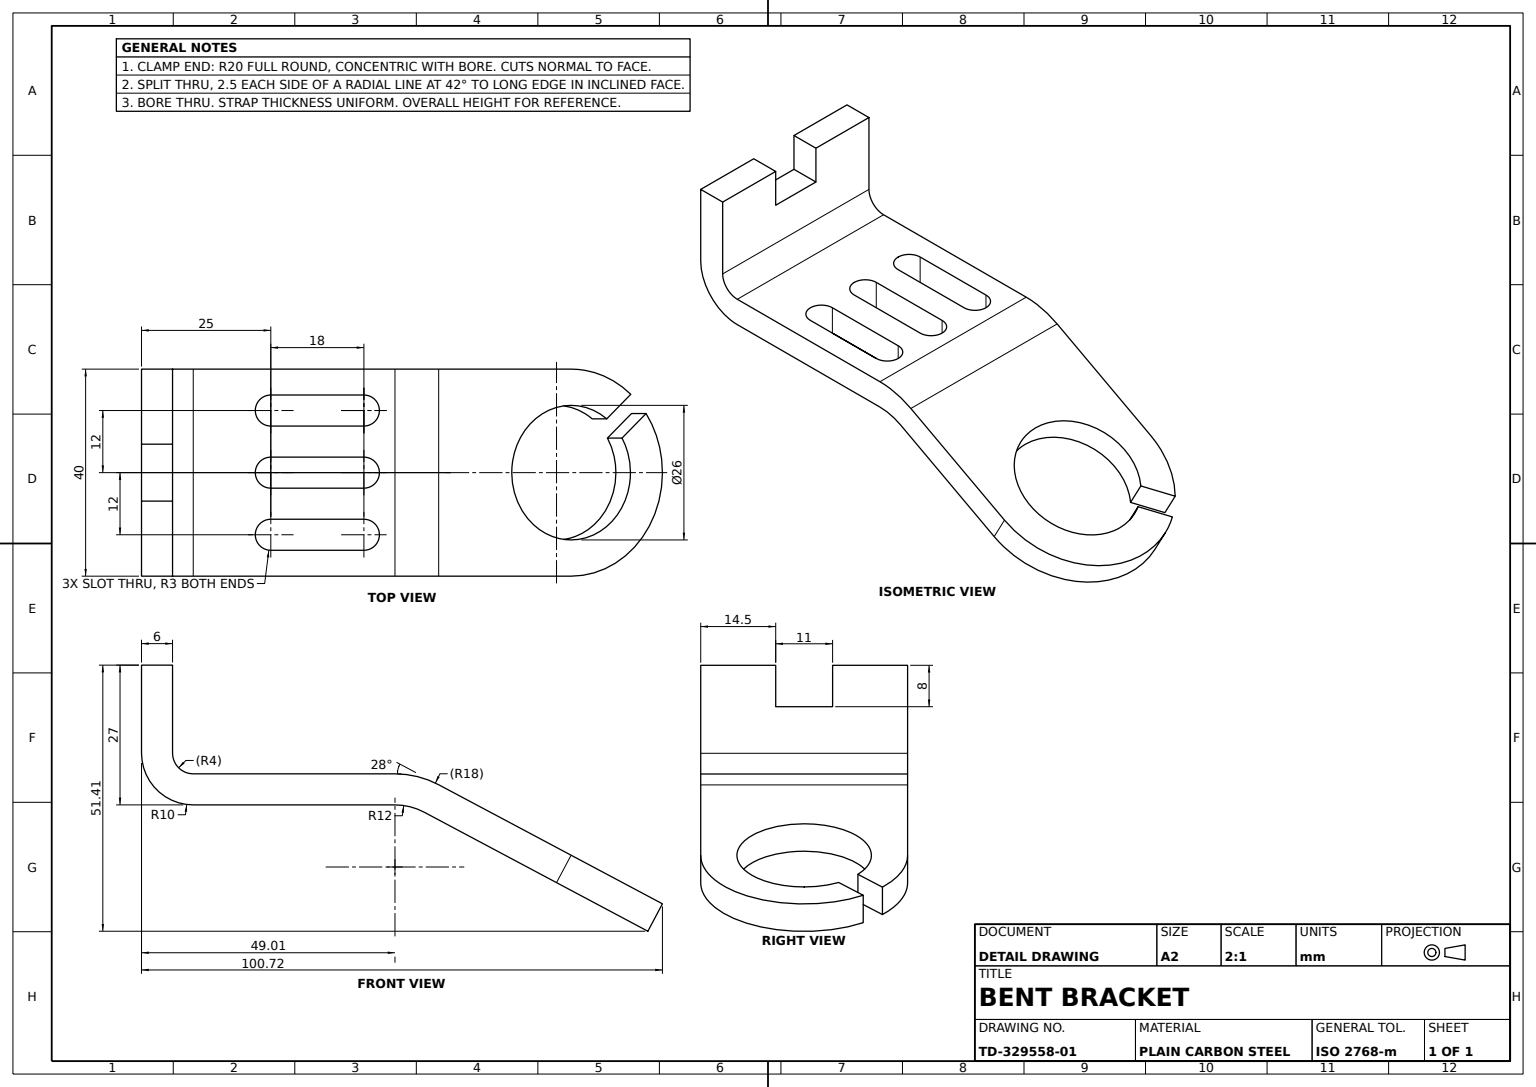
SolidWorks part; units mm, degrees
material "Plain Carbon Steel"
ref_plane "Front Plane" through (0, 0, 0) normal (0, 0, 1) x (1, 0, 0)
ref_plane "Top Plane" through (0, 0, 0) normal (0, 1, 0) x (1, 0, 0)
ref_plane "Right Plane" through (0, 0, 0) normal (1, 0, 0) x (0, 0, -1)
sketch "Strap Profile Sketch" plane through (0, 0, 0) normal (0, 0, 1) x (1, 0, 0)
  line L0 (0, 27) -> (0, 10)
  line L1 (10, 0) -> (49.0081, 0)
  line L2 (54.6417, -1.4046) -> (102, -26.5855)
  line L3 (6, 27) -> (6, 10)
  line L4 (10, 6) -> (49.0081, 6)
  line L5 (57.4586, 3.8931) -> (104.8168, -21.2878)
  line L6 (0, 27) -> (6, 27)
  line L7 (104.8168, -21.2878) -> (102, -26.5855)
  arc A0 (0, 10) -> (10, 0) centre (10, 10) ccw
  arc A1 (49.0081, 0) -> (54.6417, -1.4046) centre (49.0081, -12) cw
  arc A2 (6, 10) -> (10, 6) centre (10, 10) ccw
  arc A3 (49.0081, 6) -> (57.4586, 3.8931) centre (49.0081, -12) cw
  point P7 (0, 0)
  point P10 (52, 0)
  dimension "D4" = 10
  dimension "D5" = 12
  dimension "D1" = 27
  dimension "D2" = 52
  dimension "D3" = 50
  dimension "D6" = 28
  dimension "D7" = 6
extrude "Bent Strap Body" add sketch "Strap Profile Sketch" along normal blind 40
sketch "Slots Sketch" plane through (0, 6, 0) normal (0, 1, 0) x (1, 0, 0)
  line L0 (25, -20) -> (43, -20) construction
  line L1 (25, -17) -> (43, -17)
  line L2 (25, -23) -> (43, -23)
  line L3 (0, -40) -> (0, 0) construction
  line L4 (25, -8) -> (43, -8) construction
  line L5 (25, -5) -> (43, -5)
  line L6 (25, -11) -> (43, -11)
  line L7 (25, -32) -> (43, -32) construction
  line L8 (25, -29) -> (43, -29)
  line L9 (25, -35) -> (43, -35)
  line L10 (49.0081, 0) -> (10, 0) construction
  arc A0 (25, -17) -> (25, -23) centre (25, -20) ccw
  arc A1 (43, -23) -> (43, -17) centre (43, -20) ccw
  arc A2 (25, -5) -> (25, -11) centre (25, -8) ccw
  arc A3 (43, -11) -> (43, -5) centre (43, -8) ccw
  arc A4 (25, -29) -> (25, -35) centre (25, -32) ccw
  arc A5 (43, -35) -> (43, -29) centre (43, -32) ccw
  point P2 (34, -20)
  point P11 (34, -8)
  point P18 (34, -32)
  dimension "D1" = 18
  dimension "D2" = 25
  dimension "D3" = 6
  dimension "D4" = 18
  dimension "D5" = 25
  dimension "D6" = 12
  dimension "D7" = 6
  dimension "D8" = 6
  dimension "D9" = 18
  dimension "D10" = 25
  dimension "D11" = 12
  dimension "D12" = 20
extrude "Slots 3x6 Wide" cut sketch "Slots Sketch" against normal up to next
sketch "Split Clamp Ring Sketch" plane through (14.2778, 26.8527, 0) normal (0.4695, 0.8829, 0) x (0.8829, -0.4695, 0)
  line L0 (48.9052, -40) -> (48.9052, 0) construction
  line L1 (48.9052, -40) -> (48.9052, 0) construction
  line L2 (102.5418, 0) -> (48.9052, 0) construction
  line L3 (77.9052, -20) -> (108.692, 7.7206) construction
  line L4 (77.9052, -20) -> (118.3656, -20) construction
  line L6 (85.7129, -9.6058) -> (90.9787, -4.8645)
  line L7 (76.2324, -18.1421) -> (107.0192, 9.5784) construction
  line L9 (89.0586, -13.3215) -> (94.3244, -8.5802)
  arc A0 (85.7129, -9.6058) -> (89.0586, -13.3215) centre (77.9052, -20) ccw
  arc A1 (90.9787, -4.8645) -> (94.3244, -8.5802) centre (77.9052, -20) ccw
  line M7 (102.5418, 0) -> (48.9052, 0)
  line M9 (48.9052, -40) -> (102.5418, -40)
  line M10 (102.5418, -40) -> (102.5418, 0)
  dimension "D1" = 26
  dimension "D4" = 40
  dimension "D2" = 29
  dimension "D3" = 20
  dimension "D5" = 42
  dimension "D6" = 40.1534
  dimension "D7" = 2.5
extrude "Split Clamp Ring Cut" cut sketch "Split Clamp Ring Sketch" against normal up to next contours A1 L6 A0 L9 M9 M10 M7
sketch "End Tab Notch Sketch" plane through (6, 0, 0) normal (1, 0, 0) x (0, 0, -1)
  line L0 (-40, 27) -> (0, 27) construction
  line L1 (-25.5, 35) -> (-14.5, 35)
  line L2 (-25.5, 35) -> (-25.5, 19)
  line L3 (-25.5, 19) -> (-14.5, 19)
  line L4 (-14.5, 35) -> (-14.5, 19)
  line L5 (-25.5, 35) -> (-14.5, 19) construction
  line L6 (-25.5, 19) -> (-14.5, 35) construction
  point P0 (-20, 27)
  dimension "D1" = 11
  dimension "D2" = 8
extrude "End Tab Notch 11x8" cut sketch "End Tab Notch Sketch" against normal up to next
